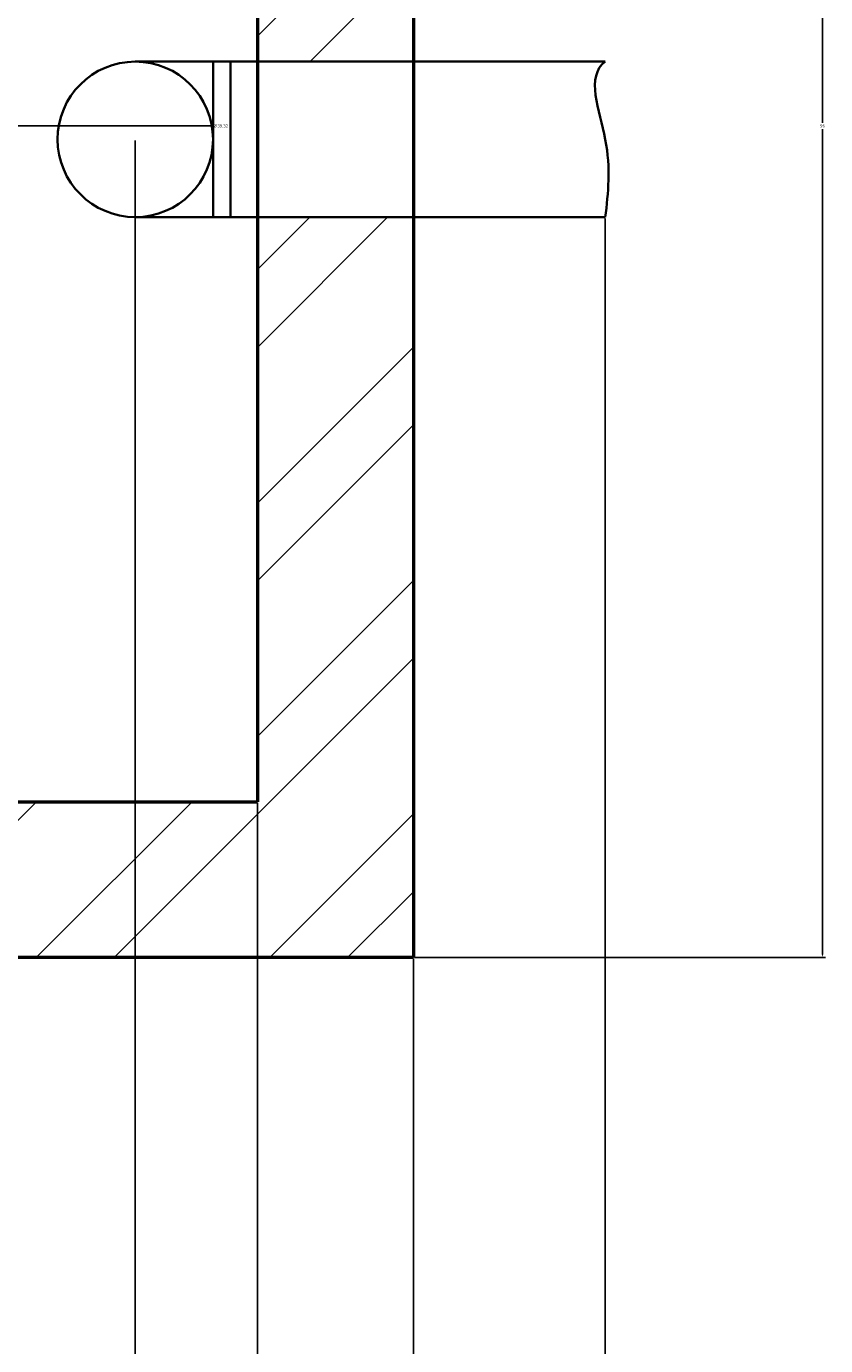
# Model space of a CAD drawing. Units: inches. Extents: x 2812 to 3051, y 1398 to 1659.
# Tile 61 of 65: x 3005 to 3051, y 1528 to 1605. Entities that reach past the tile are written whole.
import ezdxf

# ---------------------------------------------------------------- set-up
doc = ezdxf.new("R2010")
doc.units = ezdxf.units.IN
for name, color, linetype, lineweight in [('A-ANNO-DIMS', 2, 'Continuous', 18), ('P-SANR-PIPE', 4, 'Continuous', 35), ('S-CONC', 7, 'Continuous', 50), ('S-CONC-PATT', 8, 'Continuous', 18)]:
    doc.layers.add(name, color=color, linetype=linetype, lineweight=lineweight)
doc.styles.get("Standard").update_dxf_attribs({"font": 'arial.ttf'})
doc.dimstyles.get("Standard").update_dxf_attribs({"dimtxt": 0.18, "dimasz": 0.18, "dimexe": 0.18, "dimexo": 0.0625, "dimgap": 0.09, "dimtad": 0, "dimtih": 1, "dimtoh": 1, "dimdec": 4, "dimzin": 0, "dimdsep": 46, "dimtxsty": 'Standard', "dimcen": 0.09, "dimadec": 0, "dimazin": 0, "dimtfac": 1, "dimtdec": 4, "dimtofl": 0, "dimtmove": 0, "dimatfit": 3, "dimfxl": 1, "dimtolj": 1, "dimtzin": 0, "dimarcsym": 0})

# ---------------------------------------------------------------- blocks, each defined once
blk = doc.blocks.new('PIPE-BREAK')
for p, q in [((27.315, 9), (0.19, 9)), ((0.19, 0), (27.315, 0))]:
    blk.add_line(p, q)
blk.add_open_spline([(0.19, 0), (0.025, 1.41), (-0.305, 4.231), (1.347, 8.126), (0.19, 9)], degree=3)
blk = doc.blocks.new('*D33')
at = {"layer": 'A-ANNO-DIMS', "color": 0, "lineweight": -2, "transparency": 16777216}
for p, q in [((3011.337, 1597.982), (3011.337, 1397.505)), ((3018.385, 1559.757), (3018.385, 1397.505)), ((3011.517, 1397.685), (3014.468, 1397.685)), ((3018.205, 1397.685), (3015.254, 1397.685))]:
    blk.add_line(p, q, dxfattribs=at)
at = {"layer": 'A-ANNO-DIMS', "color": 0, "transparency": 16777216}
for points in [[(3011.517, 1397.715), (3011.517, 1397.655), (3011.337, 1397.685)], [(3018.205, 1397.715), (3018.205, 1397.655), (3018.385, 1397.685)]]:
    blk.add_solid(points, dxfattribs=at)
at = {"layer": 'Defpoints', "color": 0, "transparency": 16777216}
for p in [(3011.337, 1598.044), (3018.385, 1559.82), (3018.385, 1397.685)]:
    blk.add_point(p, dxfattribs=at)
at = {"layer": 'A-ANNO-DIMS', "color": 0, "transparency": 16777216, "insert": (3014.861, 1397.685), "char_height": 0.18, "attachment_point": 5}
blk.add_mtext('\\A1;7.048', dxfattribs=at)
blk = doc.blocks.new('*D34')
at = {"layer": 'A-ANNO-DIMS', "color": 0, "lineweight": -2, "transparency": 16777216}
for p, q in [((3038.462, 1593.482), (3038.462, 1397.505)), ((3027.385, 1550.757), (3027.385, 1397.505)), ((3027.565, 1397.685), (3032.468, 1397.685)), ((3038.282, 1397.685), (3033.379, 1397.685))]:
    blk.add_line(p, q, dxfattribs=at)
at = {"layer": 'A-ANNO-DIMS', "color": 0, "transparency": 16777216}
for points in [[(3027.565, 1397.715), (3027.565, 1397.655), (3027.385, 1397.685)], [(3038.282, 1397.715), (3038.282, 1397.655), (3038.462, 1397.685)]]:
    blk.add_solid(points, dxfattribs=at)
at = {"layer": 'Defpoints', "color": 0, "transparency": 16777216}
for p in [(3038.462, 1593.544), (3027.385, 1550.82), (3038.462, 1397.685)]:
    blk.add_point(p, dxfattribs=at)
at = {"layer": 'A-ANNO-DIMS', "color": 0, "transparency": 16777216, "insert": (3032.923, 1397.685), "char_height": 0.18, "attachment_point": 5}
blk.add_mtext('\\A1;11.077', dxfattribs=at)
blk = doc.blocks.new('*D35')
at = {"layer": 'A-ANNO-DIMS', "color": 0, "lineweight": -2, "transparency": 16777216}
for p, q in [((3027.447, 1646.82), (3051.178, 1646.82)), ((3050.998, 1646.64), (3050.998, 1599.002)), ((3050.998, 1551), (3050.998, 1598.638)), ((3027.447, 1550.82), (3051.178, 1550.82))]:
    blk.add_line(p, q, dxfattribs=at)
at = {"layer": 'A-ANNO-DIMS', "color": 0, "transparency": 16777216}
for points in [[(3050.968, 1646.64), (3051.028, 1646.64), (3050.998, 1646.82)], [(3050.968, 1551), (3051.028, 1551), (3050.998, 1550.82)]]:
    blk.add_solid(points, dxfattribs=at)
at = {"layer": 'Defpoints', "color": 0, "transparency": 16777216}
for p in [(3027.385, 1646.82), (3050.998, 1646.82), (3027.385, 1550.82)]:
    blk.add_point(p, dxfattribs=at)
at = {"layer": 'A-ANNO-DIMS', "color": 0, "transparency": 16777216, "insert": (3050.998, 1598.82), "char_height": 0.18, "attachment_point": 5}
blk.add_mtext('\\A1;96', dxfattribs=at)
blk = doc.blocks.new('*D83')
at = {"layer": 'A-ANNO-DIMS', "color": 0, "lineweight": -2, "transparency": 16777216}
for p, q in [((2984.316, 1598.73), (2984.316, 1598.91)), ((2984.226, 1598.82), (2984.406, 1598.82)), ((3015.77, 1598.82), (3004.154, 1598.82))]:
    blk.add_line(p, q, dxfattribs=at)
at = {"layer": 'A-ANNO-DIMS', "color": 0, "transparency": 16777216}
blk.add_solid([(3004.154, 1598.85), (3004.154, 1598.79), (3003.974, 1598.82)], dxfattribs=at)
at = {"layer": 'Defpoints', "color": 0, "transparency": 16777216}
for p in [(2964.657, 1598.82), (3003.974, 1598.82)]:
    blk.add_point(p, dxfattribs=at)
at = {"layer": 'A-ANNO-DIMS', "color": 0, "transparency": 16777216, "insert": (3016.26, 1598.82), "char_height": 0.18, "attachment_point": 5}
blk.add_mtext('\\A1;∅39.32', dxfattribs=at)

msp = doc.modelspace()

# ---------------------------------------------------------------- hatches: boundary and pattern name
at = {"layer": 'S-CONC-PATT'}
h = msp.add_hatch(dxfattribs=at)
h.set_pattern_fill('ANSI32', color=256)
h.paths.add_polyline_path([(3027.3849, 1646.82), (2835.3849, 1646.82), (2835.3849, 1603.2296), (2844.3849, 1603.2296), (2844.3849, 1637.82), (3018.3849, 1637.82), (3018.3849, 1602.5441), (3027.3849, 1602.5441)])
h.paths.add_polyline_path([(2844.3849, 1594.2296), (2835.3849, 1594.2296), (2835.3849, 1550.82), (3027.3849, 1550.82), (3027.3849, 1593.5441), (3018.3849, 1593.5441), (3018.3849, 1559.82), (2844.3849, 1559.82)])
h.paths.add_polyline_path([(2844.3849, 1482.0354), (2835.3849, 1482.0354), (2835.3849, 1463.4959), (2844.3849, 1463.4959)])
h.paths.add_polyline_path([(2844.3849, 1461.4959), (2835.3849, 1461.4959), (2835.3849, 1416.0354), (2844.3849, 1416.0354)])
h.paths.add_polyline_path([(3027.3849, 1482.0354), (3018.3849, 1482.0354), (3018.3849, 1463.2854), (3027.3849, 1463.2854)])
h.paths.add_polyline_path([(3027.3849, 1461.2854), (3018.3849, 1461.2854), (3018.3849, 1416.0354), (3027.3849, 1416.0354)])
h.paths.add_polyline_path([(2961.3849, 1448.4738), (2952.3849, 1448.4738), (2952.3849, 1416.0354), (2961.3849, 1416.0354)])
h.paths.add_polyline_path([(2961.3849, 1462.3026), (2952.3849, 1462.3026), (2952.3849, 1450.4738), (2961.3849, 1450.4738)])
h.paths.add_polyline_path([(2961.3849, 1472.0354), (2952.3849, 1472.0354), (2952.3849, 1462.3026), (2961.3849, 1462.3026)])

# ---------------------------------------------------------------- linework, layer by layer
at = {"layer": 'P-SANR-PIPE'}
for p, q in [((3015.824, 1593.5441), (3015.824, 1602.5441)), ((3016.824, 1602.5441), (3016.824, 1593.5441))]:
    msp.add_line(p, q, dxfattribs=at)
msp.add_circle((3011.3373, 1598.0441), 4.4867, dxfattribs=at)
at = {"layer": 'S-CONC'}
for p, q in [((3027.3849, 1646.82), (3027.3849, 1550.82)), ((3018.3849, 1637.82), (3018.3849, 1559.82)), ((2844.3849, 1559.82), (3018.3849, 1559.82)), ((3027.3849, 1550.82), (2835.3849, 1550.82))]:
    msp.add_line(p, q, dxfattribs=at)

# ---------------------------------------------------------------- block references
at = {"layer": 'P-SANR-PIPE', "extrusion": (0, 0, -1), "zscale": -1}
msp.add_blockref('PIPE-BREAK', (-3038.6525, 1593.5445), dxfattribs=at)

# ---------------------------------------------------------------- dimensions: what is measured, and where the dimension line sits
at = {"layer": 'A-ANNO-DIMS'}
dim = msp.add_linear_dim(base=(3050.998, 1646.82), p1=(3027.3849, 1550.82), p2=(3027.3849, 1646.82), angle=90, dimstyle='Standard', override={"dimdec": 0, "dimlfac": 1, "dimrnd": 0, "dimzin": 0, "dimdsep": 46, "dimlunit": 2}, dxfattribs=at)
dim.commit()
dim.dimension.update_dxf_attribs({"geometry": '*D35', "text_midpoint": (3050.998, 1598.82)})
dim = msp.add_diameter_dim_2p(p1=(2964.6569, 1598.8199), p2=(3003.9744, 1598.82), dimstyle='Standard', override={"dimdec": 2, "dimlfac": 1, "dimrnd": 0, "dimzin": 0, "dimdsep": 46, "dimlunit": 2}, dxfattribs=at)
dim.commit()
dim.dimension.update_dxf_attribs({"geometry": '*D83', "text_midpoint": (3015.7697, 1598.82), "dimtype": 163})
for base, p1, p2, picture, middle in [((3018.3849, 1397.6854), (3011.3373, 1598.0441), (3018.3849, 1559.82), '*D33', (3014.8611, 1397.6854)), ((3038.4621, 1397.6854), (3027.3849, 1550.82), (3038.4621, 1593.5441), '*D34', (3032.9235, 1397.6854))]:
    dim = msp.add_linear_dim(base=base, p1=p1, p2=p2, dimstyle='Standard', override={"dimdec": 3, "dimlfac": 1, "dimrnd": 0, "dimzin": 0, "dimdsep": 46, "dimlunit": 2}, dxfattribs=at)
    dim.commit()
    dim.dimension.update_dxf_attribs({"geometry": picture, "text_midpoint": middle})

doc.saveas('drawing.dxf')
